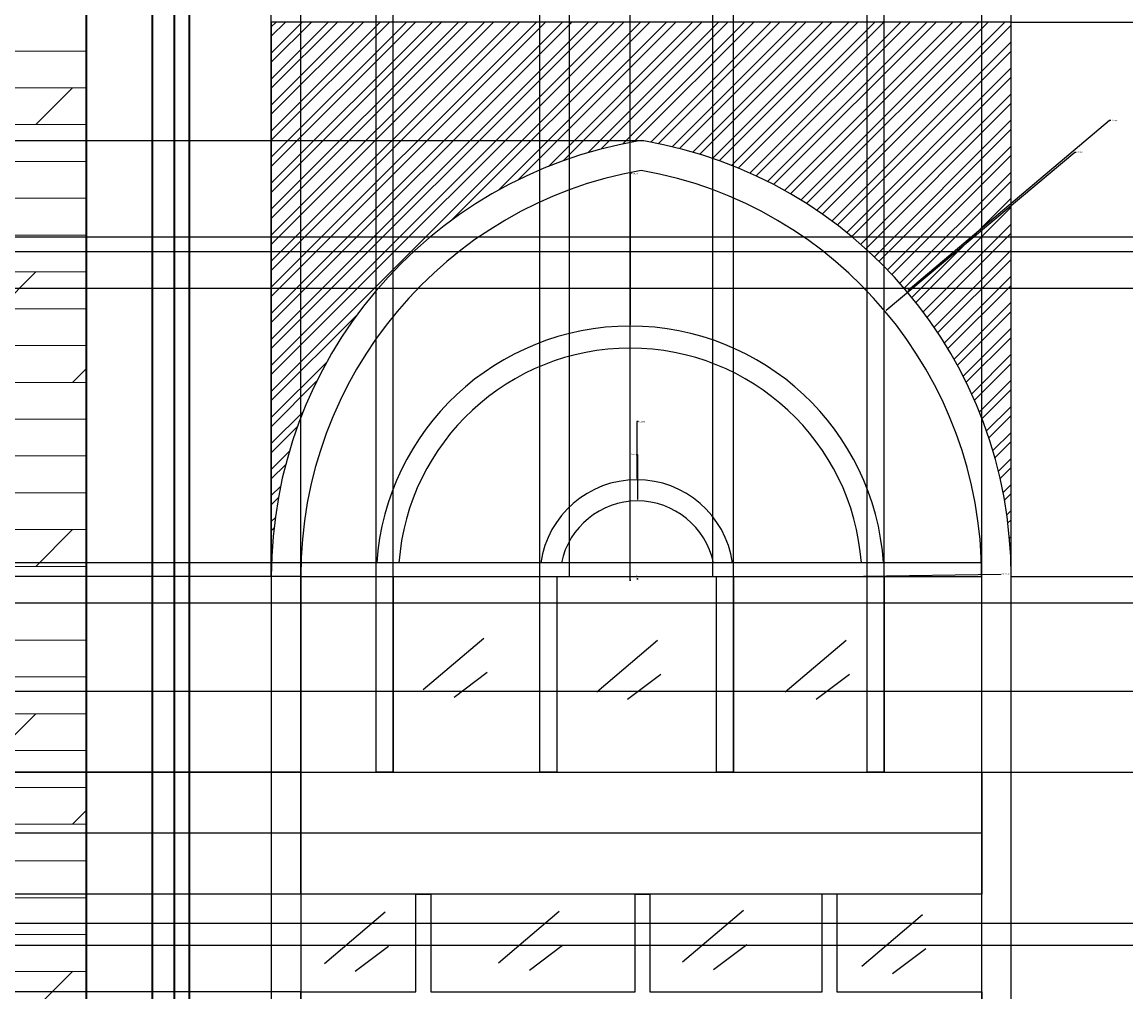
# Model space of a CAD drawing. Units: inches. Extents: x -13 to 630, y -103 to 275.
# Tile 6 of 9: x 168 to 318, y 72 to 204. Entities that reach past the tile are written whole.
import ezdxf

# ---------------------------------------------------------------- set-up
doc = ezdxf.new("R2010")
doc.units = ezdxf.units.IN
doc.header["$MEASUREMENT"] = 0
for name, color, linetype, lineweight in [('A-ANNO-DIMS', 2, 'Continuous', 18), ('A-ELEV', 7, 'Continuous', 35), ('A-ELEV-PATT', 8, 'Continuous', 13), ('A-GLAZ', 4, 'Continuous', 25)]:
    doc.layers.add(name, color=color, linetype=linetype, lineweight=lineweight)
doc.styles.get("Standard").update_dxf_attribs({"font": 'arial.ttf'})
doc.dimstyles.get("Standard").update_dxf_attribs({"dimtxt": 0.18, "dimasz": 0.18, "dimexe": 0.18, "dimexo": 0.0625, "dimgap": 0.09, "dimtad": 0, "dimtih": 1, "dimtoh": 1, "dimdec": 4, "dimzin": 0, "dimdsep": 46, "dimtxsty": 'Standard', "dimcen": 0.09, "dimadec": 0, "dimazin": 0, "dimtfac": 1, "dimtdec": 4, "dimtofl": 0, "dimtmove": 0, "dimatfit": 3, "dimfxl": 1, "dimtolj": 1, "dimtzin": 0, "dimarcsym": 0})

# ---------------------------------------------------------------- blocks, each defined once
blk = doc.blocks.new('GLAZ-MARK')
for p, q in [((0, 1.02), (8.26, 8.03)), ((4.19, 0), (8.71, 3.39))]:
    blk.add_line(p, q)
blk = doc.blocks.new('*D28')
at = {"layer": 'A-ANNO-DIMS', "color": 0, "lineweight": -2, "transparency": 16777216}
for p, q in [((302.59, 128.66), (630.03, 128.66)), ((629.85, 128.48), (629.85, 67.05)), ((629.85, 5.26), (629.85, 66.69)), ((302.59, 5.08), (630.03, 5.08))]:
    blk.add_line(p, q, dxfattribs=at)
at = {"layer": 'A-ANNO-DIMS', "color": 0, "transparency": 16777216}
for points in [[(629.82, 128.48), (629.88, 128.48), (629.85, 128.66)], [(629.82, 5.26), (629.88, 5.26), (629.85, 5.08)]]:
    blk.add_solid(points, dxfattribs=at)
at = {"layer": 'Defpoints', "color": 0, "transparency": 16777216}
for p in [(302.53, 128.66), (629.85, 128.66), (302.53, 5.08)]:
    blk.add_point(p, dxfattribs=at)
at = {"layer": 'A-ANNO-DIMS', "color": 0, "transparency": 16777216, "insert": (629.85, 66.87), "char_height": 0.18, "attachment_point": 5}
blk.add_mtext('\\A1;123.57', dxfattribs=at)
blk = doc.blocks.new('*D29')
at = {"layer": 'A-ANNO-DIMS', "color": 0, "lineweight": -2, "transparency": 16777216}
for p, q in [((302.59, 203.94), (630.03, 203.94)), ((629.85, 203.76), (629.85, 166.48)), ((629.85, 128.84), (629.85, 166.11)), ((302.59, 128.66), (630.03, 128.66))]:
    blk.add_line(p, q, dxfattribs=at)
at = {"layer": 'A-ANNO-DIMS', "color": 0, "transparency": 16777216}
for points in [[(629.82, 203.76), (629.88, 203.76), (629.85, 203.94)], [(629.82, 128.84), (629.88, 128.84), (629.85, 128.66)]]:
    blk.add_solid(points, dxfattribs=at)
at = {"layer": 'Defpoints', "color": 0, "transparency": 16777216}
for p in [(302.53, 203.94), (629.85, 203.94), (302.53, 128.66)]:
    blk.add_point(p, dxfattribs=at)
at = {"layer": 'A-ANNO-DIMS', "color": 0, "transparency": 16777216, "insert": (629.85, 166.3), "char_height": 0.18, "attachment_point": 5}
blk.add_mtext('\\A1;75.28', dxfattribs=at)
blk = doc.blocks.new('*D41')
at = {"layer": 'A-ANNO-DIMS', "color": 0, "lineweight": -2, "transparency": 16777216}
for p, q in [((205.96, 72.22), (-13.22, 72.22)), ((-13.04, 72.04), (-13.04, 71.07)), ((-13.04, 69.73), (-13.04, 70.7)), ((205.96, 69.55), (-13.22, 69.55))]:
    blk.add_line(p, q, dxfattribs=at)
at = {"layer": 'A-ANNO-DIMS', "color": 0, "transparency": 16777216}
for points in [[(-13.07, 72.04), (-13.01, 72.04), (-13.04, 72.22)], [(-13.07, 69.73), (-13.01, 69.73), (-13.04, 69.55)]]:
    blk.add_solid(points, dxfattribs=at)
at = {"layer": 'Defpoints', "color": 0, "transparency": 16777216}
for p in [(-13.04, 72.22), (206.02, 72.22), (206.02, 69.55)]:
    blk.add_point(p, dxfattribs=at)
at = {"layer": 'A-ANNO-DIMS', "color": 0, "transparency": 16777216, "insert": (-13.04, 70.88), "char_height": 0.18, "attachment_point": 5}
blk.add_mtext('\\A1;2.68', dxfattribs=at)
blk = doc.blocks.new('*D42')
at = {"layer": 'A-ANNO-DIMS', "color": 0, "lineweight": -2, "transparency": 16777216}
for p, q in [((205.96, 85.52), (-13.22, 85.52)), ((-13.04, 85.34), (-13.04, 79.05)), ((-13.04, 72.4), (-13.04, 78.69)), ((205.96, 72.22), (-13.22, 72.22))]:
    blk.add_line(p, q, dxfattribs=at)
at = {"layer": 'A-ANNO-DIMS', "color": 0, "transparency": 16777216}
for points in [[(-13.07, 85.34), (-13.01, 85.34), (-13.04, 85.52)], [(-13.07, 72.4), (-13.01, 72.4), (-13.04, 72.22)]]:
    blk.add_solid(points, dxfattribs=at)
at = {"layer": 'Defpoints', "color": 0, "transparency": 16777216}
for p in [(-13.04, 85.52), (206.02, 85.52), (206.02, 72.22)]:
    blk.add_point(p, dxfattribs=at)
at = {"layer": 'A-ANNO-DIMS', "color": 0, "transparency": 16777216, "insert": (-13.04, 78.87), "char_height": 0.18, "attachment_point": 5}
blk.add_mtext('\\A1;13.297', dxfattribs=at)
blk = doc.blocks.new('*D43')
at = {"layer": 'A-ANNO-DIMS', "color": 0, "lineweight": -2, "transparency": 16777216}
for p, q in [((205.96, 93.8), (-13.22, 93.8)), ((-13.04, 93.62), (-13.04, 89.84)), ((-13.04, 85.7), (-13.04, 89.48)), ((205.96, 85.52), (-13.22, 85.52))]:
    blk.add_line(p, q, dxfattribs=at)
at = {"layer": 'A-ANNO-DIMS', "color": 0, "transparency": 16777216}
for points in [[(-13.07, 93.62), (-13.01, 93.62), (-13.04, 93.8)], [(-13.07, 85.7), (-13.01, 85.7), (-13.04, 85.52)]]:
    blk.add_solid(points, dxfattribs=at)
at = {"layer": 'Defpoints', "color": 0, "transparency": 16777216}
for p in [(-13.04, 93.8), (206.02, 93.8), (206.02, 85.52)]:
    blk.add_point(p, dxfattribs=at)
at = {"layer": 'A-ANNO-DIMS', "color": 0, "transparency": 16777216, "insert": (-13.04, 89.66), "char_height": 0.18, "attachment_point": 5}
blk.add_mtext('\\A1;8.28', dxfattribs=at)
blk = doc.blocks.new('*D44')
at = {"layer": 'A-ANNO-DIMS', "color": 0, "lineweight": -2, "transparency": 16777216}
for p, q in [((205.96, 102.08), (-13.22, 102.08)), ((-13.04, 101.9), (-13.04, 98.12)), ((-13.04, 93.98), (-13.04, 97.76)), ((205.96, 93.8), (-13.22, 93.8))]:
    blk.add_line(p, q, dxfattribs=at)
at = {"layer": 'A-ANNO-DIMS', "color": 0, "transparency": 16777216}
for points in [[(-13.07, 101.9), (-13.01, 101.9), (-13.04, 102.08)], [(-13.07, 93.98), (-13.01, 93.98), (-13.04, 93.8)]]:
    blk.add_solid(points, dxfattribs=at)
at = {"layer": 'Defpoints', "color": 0, "transparency": 16777216}
for p in [(-13.04, 102.08), (206.02, 102.08), (206.02, 93.8)]:
    blk.add_point(p, dxfattribs=at)
at = {"layer": 'A-ANNO-DIMS', "color": 0, "transparency": 16777216, "insert": (-13.04, 97.94), "char_height": 0.18, "attachment_point": 5}
blk.add_mtext('\\A1;8.28', dxfattribs=at)
blk = doc.blocks.new('*D45')
at = {"layer": 'A-ANNO-DIMS', "color": 0, "lineweight": -2, "transparency": 16777216}
for p, q in [((205.96, 128.66), (-13.22, 128.66)), ((-13.04, 128.48), (-13.04, 115.55)), ((-13.04, 102.26), (-13.04, 115.19)), ((205.96, 102.08), (-13.22, 102.08))]:
    blk.add_line(p, q, dxfattribs=at)
at = {"layer": 'A-ANNO-DIMS', "color": 0, "transparency": 16777216}
for points in [[(-13.07, 128.48), (-13.01, 128.48), (-13.04, 128.66)], [(-13.07, 102.26), (-13.01, 102.26), (-13.04, 102.08)]]:
    blk.add_solid(points, dxfattribs=at)
at = {"layer": 'Defpoints', "color": 0, "transparency": 16777216}
for p in [(-13.04, 128.66), (206.02, 128.66), (206.02, 102.08)]:
    blk.add_point(p, dxfattribs=at)
at = {"layer": 'A-ANNO-DIMS', "color": 0, "transparency": 16777216, "insert": (-13.04, 115.37), "char_height": 0.18, "attachment_point": 5}
blk.add_mtext('\\A1;26.574', dxfattribs=at)
blk = doc.blocks.new('*D46')
at = {"layer": 'A-ANNO-DIMS', "color": 0, "lineweight": -2, "transparency": 16777216}
for p, q in [((205.96, 130.51), (-13.22, 130.51)), ((-13.04, 130.33), (-13.04, 129.76)), ((-13.04, 128.84), (-13.04, 129.4)), ((205.96, 128.66), (-13.22, 128.66))]:
    blk.add_line(p, q, dxfattribs=at)
at = {"layer": 'A-ANNO-DIMS', "color": 0, "transparency": 16777216}
for points in [[(-13.07, 130.33), (-13.01, 130.33), (-13.04, 130.51)], [(-13.07, 128.84), (-13.01, 128.84), (-13.04, 128.66)]]:
    blk.add_solid(points, dxfattribs=at)
at = {"layer": 'Defpoints', "color": 0, "transparency": 16777216}
for p in [(-13.04, 130.51), (206.02, 130.51), (206.02, 128.66)]:
    blk.add_point(p, dxfattribs=at)
at = {"layer": 'A-ANNO-DIMS', "color": 0, "transparency": 16777216, "insert": (-13.04, 129.58), "char_height": 0.18, "attachment_point": 5}
blk.add_mtext('\\A1;1.854', dxfattribs=at)
blk = doc.blocks.new('*D47')
at = {"layer": 'A-ANNO-DIMS', "color": 0, "lineweight": -2, "transparency": 16777216}
for p, q in [((252.21, 187.83), (-13.22, 187.83)), ((-13.04, 187.65), (-13.04, 159.35)), ((-13.04, 130.69), (-13.04, 158.99)), ((205.96, 130.51), (-13.22, 130.51))]:
    blk.add_line(p, q, dxfattribs=at)
at = {"layer": 'A-ANNO-DIMS', "color": 0, "transparency": 16777216}
for points in [[(-13.07, 187.65), (-13.01, 187.65), (-13.04, 187.83)], [(-13.07, 130.69), (-13.01, 130.69), (-13.04, 130.51)]]:
    blk.add_solid(points, dxfattribs=at)
at = {"layer": 'Defpoints', "color": 0, "transparency": 16777216}
for p in [(-13.04, 187.83), (252.27, 187.83), (206.02, 130.51)]:
    blk.add_point(p, dxfattribs=at)
at = {"layer": 'A-ANNO-DIMS', "color": 0, "transparency": 16777216, "insert": (-13.04, 159.17), "char_height": 0.18, "attachment_point": 5}
blk.add_mtext('\\A1;57.32', dxfattribs=at)
blk = doc.blocks.new('*D56')
at = {"layer": 'A-ANNO-DIMS', "color": 0, "lineweight": -2, "transparency": 16777216}
for p, q in [((206.02, 102.14), (206.02, 275.01)), ((206.2, 274.83), (210.69, 274.83)), ((216.09, 274.83), (211.6, 274.83)), ((216.27, 102.14), (216.27, 275.01))]:
    blk.add_line(p, q, dxfattribs=at)
at = {"layer": 'A-ANNO-DIMS', "color": 0, "transparency": 16777216}
for points in [[(206.2, 274.86), (206.2, 274.8), (206.02, 274.83)], [(216.09, 274.86), (216.09, 274.8), (216.27, 274.83)]]:
    blk.add_solid(points, dxfattribs=at)
at = {"layer": 'Defpoints', "color": 0, "transparency": 16777216}
for p in [(216.27, 274.83), (206.02, 102.08), (216.27, 102.08)]:
    blk.add_point(p, dxfattribs=at)
at = {"layer": 'A-ANNO-DIMS', "color": 0, "transparency": 16777216, "insert": (211.14, 274.83), "char_height": 0.18, "attachment_point": 5}
blk.add_mtext('\\A1;10.246', dxfattribs=at)
blk = doc.blocks.new('*D57')
at = {"layer": 'A-ANNO-DIMS', "color": 0, "lineweight": -2, "transparency": 16777216}
for p, q in [((216.27, 102.14), (216.27, 275.01)), ((216.45, 274.83), (217.02, 274.83)), ((218.38, 274.83), (217.81, 274.83)), ((218.56, 102.14), (218.56, 275.01))]:
    blk.add_line(p, q, dxfattribs=at)
at = {"layer": 'A-ANNO-DIMS', "color": 0, "transparency": 16777216}
for points in [[(216.45, 274.86), (216.45, 274.8), (216.27, 274.83)], [(218.38, 274.86), (218.38, 274.8), (218.56, 274.83)]]:
    blk.add_solid(points, dxfattribs=at)
at = {"layer": 'Defpoints', "color": 0, "transparency": 16777216}
for p in [(218.56, 274.83), (216.27, 102.08), (218.56, 102.08)]:
    blk.add_point(p, dxfattribs=at)
at = {"layer": 'A-ANNO-DIMS', "color": 0, "transparency": 16777216, "insert": (217.42, 274.83), "char_height": 0.18, "attachment_point": 5}
blk.add_mtext('\\A1;2.298', dxfattribs=at)
blk = doc.blocks.new('*D58')
at = {"layer": 'A-ANNO-DIMS', "color": 0, "lineweight": -2, "transparency": 16777216}
for p, q in [((218.56, 102.14), (218.56, 275.01)), ((218.74, 274.83), (228.14, 274.83)), ((238.31, 274.83), (228.91, 274.83)), ((238.49, 102.14), (238.49, 275.01))]:
    blk.add_line(p, q, dxfattribs=at)
at = {"layer": 'A-ANNO-DIMS', "color": 0, "transparency": 16777216}
for points in [[(218.74, 274.86), (218.74, 274.8), (218.56, 274.83)], [(238.31, 274.86), (238.31, 274.8), (238.49, 274.83)]]:
    blk.add_solid(points, dxfattribs=at)
at = {"layer": 'Defpoints', "color": 0, "transparency": 16777216}
for p in [(238.49, 274.83), (218.56, 102.08), (238.49, 102.08)]:
    blk.add_point(p, dxfattribs=at)
at = {"layer": 'A-ANNO-DIMS', "color": 0, "transparency": 16777216, "insert": (228.53, 274.83), "char_height": 0.18, "attachment_point": 5}
blk.add_mtext('\\A1;19.93', dxfattribs=at)
blk = doc.blocks.new('*D59')
at = {"layer": 'A-ANNO-DIMS', "color": 0, "lineweight": -2, "transparency": 16777216}
for p, q in [((238.49, 102.14), (238.49, 275.01)), ((238.67, 274.83), (251.26, 274.83)), ((264.64, 274.83), (252.05, 274.83)), ((264.82, 102.14), (264.82, 275.01))]:
    blk.add_line(p, q, dxfattribs=at)
at = {"layer": 'A-ANNO-DIMS', "color": 0, "transparency": 16777216}
for points in [[(238.67, 274.86), (238.67, 274.8), (238.49, 274.83)], [(264.64, 274.86), (264.64, 274.8), (264.82, 274.83)]]:
    blk.add_solid(points, dxfattribs=at)
at = {"layer": 'Defpoints', "color": 0, "transparency": 16777216}
for p in [(264.82, 274.83), (238.49, 102.08), (264.82, 102.08)]:
    blk.add_point(p, dxfattribs=at)
at = {"layer": 'A-ANNO-DIMS', "color": 0, "transparency": 16777216, "insert": (251.66, 274.83), "char_height": 0.18, "attachment_point": 5}
blk.add_mtext('\\A1;26.32', dxfattribs=at)
blk = doc.blocks.new('*D60')
at = {"layer": 'A-ANNO-DIMS', "color": 0, "lineweight": -2, "transparency": 16777216}
for p, q in [((264.82, 102.14), (264.82, 275.01)), ((265, 274.83), (273.44, 274.83)), ((282.8, 274.83), (274.35, 274.83)), ((282.98, 102.14), (282.98, 275.01))]:
    blk.add_line(p, q, dxfattribs=at)
at = {"layer": 'A-ANNO-DIMS', "color": 0, "transparency": 16777216}
for points in [[(265, 274.86), (265, 274.8), (264.82, 274.83)], [(282.8, 274.86), (282.8, 274.8), (282.98, 274.83)]]:
    blk.add_solid(points, dxfattribs=at)
at = {"layer": 'Defpoints', "color": 0, "transparency": 16777216}
for p in [(282.98, 274.83), (264.82, 102.08), (282.98, 102.08)]:
    blk.add_point(p, dxfattribs=at)
at = {"layer": 'A-ANNO-DIMS', "color": 0, "transparency": 16777216, "insert": (273.9, 274.83), "char_height": 0.18, "attachment_point": 5}
blk.add_mtext('\\A1;18.158', dxfattribs=at)
blk = doc.blocks.new('*D61')
at = {"layer": 'A-ANNO-DIMS', "color": 0, "lineweight": -2, "transparency": 16777216}
for p, q in [((282.98, 102.14), (282.98, 275.01)), ((283.16, 274.83), (283.73, 274.83)), ((285.09, 274.83), (284.52, 274.83)), ((285.27, 102.14), (285.27, 275.01))]:
    blk.add_line(p, q, dxfattribs=at)
at = {"layer": 'A-ANNO-DIMS', "color": 0, "transparency": 16777216}
for points in [[(283.16, 274.86), (283.16, 274.8), (282.98, 274.83)], [(285.09, 274.86), (285.09, 274.8), (285.27, 274.83)]]:
    blk.add_solid(points, dxfattribs=at)
at = {"layer": 'Defpoints', "color": 0, "transparency": 16777216}
for p in [(285.27, 274.83), (282.98, 102.08), (285.27, 102.08)]:
    blk.add_point(p, dxfattribs=at)
at = {"layer": 'A-ANNO-DIMS', "color": 0, "transparency": 16777216, "insert": (284.12, 274.83), "char_height": 0.18, "attachment_point": 5}
blk.add_mtext('\\A1;2.298', dxfattribs=at)
blk = doc.blocks.new('*D62')
at = {"layer": 'A-ANNO-DIMS', "color": 0, "lineweight": -2, "transparency": 16777216}
for p, q in [((285.27, 102.14), (285.27, 275.01)), ((285.45, 274.83), (291.44, 274.83)), ((298.35, 274.83), (292.35, 274.83)), ((298.53, 102.14), (298.53, 275.01))]:
    blk.add_line(p, q, dxfattribs=at)
at = {"layer": 'A-ANNO-DIMS', "color": 0, "transparency": 16777216}
for points in [[(285.45, 274.86), (285.45, 274.8), (285.27, 274.83)], [(298.35, 274.86), (298.35, 274.8), (298.53, 274.83)]]:
    blk.add_solid(points, dxfattribs=at)
at = {"layer": 'Defpoints', "color": 0, "transparency": 16777216}
for p in [(298.53, 274.83), (285.27, 102.08), (298.53, 102.08)]:
    blk.add_point(p, dxfattribs=at)
at = {"layer": 'A-ANNO-DIMS', "color": 0, "transparency": 16777216, "insert": (291.9, 274.83), "char_height": 0.18, "attachment_point": 5}
blk.add_mtext('\\A1;13.253', dxfattribs=at)
blk = doc.blocks.new('*D63')
at = {"layer": 'A-ANNO-DIMS', "color": 0, "lineweight": -2, "transparency": 16777216}
for p, q in [((202.02, 128.72), (202.02, 275.01)), ((202.2, 274.83), (221.81, 274.83)), ((242.35, 274.83), (222.74, 274.83)), ((242.53, 128.72), (242.53, 275.01))]:
    blk.add_line(p, q, dxfattribs=at)
at = {"layer": 'A-ANNO-DIMS', "color": 0, "transparency": 16777216}
for points in [[(202.2, 274.86), (202.2, 274.8), (202.02, 274.83)], [(242.35, 274.86), (242.35, 274.8), (242.53, 274.83)]]:
    blk.add_solid(points, dxfattribs=at)
at = {"layer": 'Defpoints', "color": 0, "transparency": 16777216}
for p in [(242.53, 274.83), (202.02, 128.66), (242.53, 128.66)]:
    blk.add_point(p, dxfattribs=at)
at = {"layer": 'A-ANNO-DIMS', "color": 0, "transparency": 16777216, "insert": (222.27, 274.83), "char_height": 0.18, "attachment_point": 5}
blk.add_mtext('\\A1;40.505', dxfattribs=at)
blk = doc.blocks.new('*D64')
at = {"layer": 'A-ANNO-DIMS', "color": 0, "lineweight": -2, "transparency": 16777216}
for p, q in [((242.53, 128.72), (242.53, 275.01)), ((242.71, 274.83), (246.25, 274.83)), ((250.59, 274.83), (247.04, 274.83)), ((250.77, 128.2), (250.77, 275.01))]:
    blk.add_line(p, q, dxfattribs=at)
at = {"layer": 'A-ANNO-DIMS', "color": 0, "transparency": 16777216}
for points in [[(242.71, 274.86), (242.71, 274.8), (242.53, 274.83)], [(250.59, 274.86), (250.59, 274.8), (250.77, 274.83)]]:
    blk.add_solid(points, dxfattribs=at)
at = {"layer": 'Defpoints', "color": 0, "transparency": 16777216}
for p in [(250.77, 274.83), (242.53, 128.66), (250.77, 128.14)]:
    blk.add_point(p, dxfattribs=at)
at = {"layer": 'A-ANNO-DIMS', "color": 0, "transparency": 16777216, "insert": (246.65, 274.83), "char_height": 0.18, "attachment_point": 5}
blk.add_mtext('\\A1;8.244', dxfattribs=at)
blk = doc.blocks.new('*D65')
at = {"layer": 'A-ANNO-DIMS', "color": 0, "lineweight": -2, "transparency": 16777216}
for p, q in [((250.77, 128.2), (250.77, 275.01)), ((250.95, 274.83), (256.01, 274.83)), ((261.84, 274.83), (256.78, 274.83)), ((262.02, 128.72), (262.02, 275.01))]:
    blk.add_line(p, q, dxfattribs=at)
at = {"layer": 'A-ANNO-DIMS', "color": 0, "transparency": 16777216}
for points in [[(250.95, 274.86), (250.95, 274.8), (250.77, 274.83)], [(261.84, 274.86), (261.84, 274.8), (262.02, 274.83)]]:
    blk.add_solid(points, dxfattribs=at)
at = {"layer": 'Defpoints', "color": 0, "transparency": 16777216}
for p in [(262.02, 274.83), (250.77, 128.14), (262.02, 128.66)]:
    blk.add_point(p, dxfattribs=at)
at = {"layer": 'A-ANNO-DIMS', "color": 0, "transparency": 16777216, "insert": (256.4, 274.83), "char_height": 0.18, "attachment_point": 5}
blk.add_mtext('\\A1;11.25', dxfattribs=at)
blk = doc.blocks.new('*D66')
at = {"layer": 'A-ANNO-DIMS', "color": 0, "lineweight": -2, "transparency": 16777216}
for p, q in [((262.02, 128.72), (262.02, 275.01)), ((262.2, 274.83), (281.81, 274.83)), ((302.35, 274.83), (282.74, 274.83)), ((302.53, 128.72), (302.53, 275.01))]:
    blk.add_line(p, q, dxfattribs=at)
at = {"layer": 'A-ANNO-DIMS', "color": 0, "transparency": 16777216}
for points in [[(262.2, 274.86), (262.2, 274.8), (262.02, 274.83)], [(302.35, 274.86), (302.35, 274.8), (302.53, 274.83)]]:
    blk.add_solid(points, dxfattribs=at)
at = {"layer": 'Defpoints', "color": 0, "transparency": 16777216}
for p in [(302.53, 274.83), (262.02, 128.66), (302.53, 128.66)]:
    blk.add_point(p, dxfattribs=at)
at = {"layer": 'A-ANNO-DIMS', "color": 0, "transparency": 16777216, "insert": (282.27, 274.83), "char_height": 0.18, "attachment_point": 5}
blk.add_mtext('\\A1;40.505', dxfattribs=at)
blk = doc.blocks.new('*D83')
at = {"layer": 'A-ANNO-DIMS', "color": 0, "lineweight": -2, "transparency": 16777216}
for p, q in [((134.77, 78.57), (630.03, 78.57)), ((629.85, 78.39), (629.85, 70.42)), ((629.85, 62.08), (629.85, 70.05)), ((134.77, 61.9), (630.03, 61.9))]:
    blk.add_line(p, q, dxfattribs=at)
at = {"layer": 'A-ANNO-DIMS', "color": 0, "transparency": 16777216}
for points in [[(629.82, 78.39), (629.88, 78.39), (629.85, 78.57)], [(629.82, 62.08), (629.88, 62.08), (629.85, 61.9)]]:
    blk.add_solid(points, dxfattribs=at)
at = {"layer": 'Defpoints', "color": 0, "transparency": 16777216}
for p in [(134.71, 78.57), (629.85, 78.57), (134.71, 61.9)]:
    blk.add_point(p, dxfattribs=at)
at = {"layer": 'A-ANNO-DIMS', "color": 0, "transparency": 16777216, "insert": (629.85, 70.24), "char_height": 0.18, "attachment_point": 5}
blk.add_mtext('\\A1;16.67', dxfattribs=at)
blk = doc.blocks.new('*D84')
at = {"layer": 'A-ANNO-DIMS', "color": 0, "lineweight": -2, "transparency": 16777216}
for p, q in [((137.77, 81.57), (630.03, 81.57)), ((629.85, 81.39), (629.85, 80.25)), ((629.85, 78.75), (629.85, 79.89)), ((134.77, 78.57), (630.03, 78.57))]:
    blk.add_line(p, q, dxfattribs=at)
at = {"layer": 'A-ANNO-DIMS', "color": 0, "transparency": 16777216}
for points in [[(629.82, 81.39), (629.88, 81.39), (629.85, 81.57)], [(629.82, 78.75), (629.88, 78.75), (629.85, 78.57)]]:
    blk.add_solid(points, dxfattribs=at)
at = {"layer": 'Defpoints', "color": 0, "transparency": 16777216}
for p in [(137.71, 81.57), (629.85, 81.57), (134.71, 78.57)]:
    blk.add_point(p, dxfattribs=at)
at = {"layer": 'A-ANNO-DIMS', "color": 0, "transparency": 16777216, "insert": (629.85, 80.07), "char_height": 0.18, "attachment_point": 5}
blk.add_mtext('\\A1;3', dxfattribs=at)
blk = doc.blocks.new('*D85')
at = {"layer": 'A-ANNO-DIMS', "color": 0, "lineweight": -2, "transparency": 16777216}
for p, q in [((137.77, 102.08), (630.03, 102.08)), ((629.85, 101.9), (629.85, 92.01)), ((629.85, 81.75), (629.85, 91.64)), ((137.77, 81.57), (630.03, 81.57))]:
    blk.add_line(p, q, dxfattribs=at)
at = {"layer": 'A-ANNO-DIMS', "color": 0, "transparency": 16777216}
for points in [[(629.82, 101.9), (629.88, 101.9), (629.85, 102.08)], [(629.82, 81.75), (629.88, 81.75), (629.85, 81.57)]]:
    blk.add_solid(points, dxfattribs=at)
at = {"layer": 'Defpoints', "color": 0, "transparency": 16777216}
for p in [(137.71, 102.08), (629.85, 102.08), (137.71, 81.57)]:
    blk.add_point(p, dxfattribs=at)
at = {"layer": 'A-ANNO-DIMS', "color": 0, "transparency": 16777216, "insert": (629.85, 91.83), "char_height": 0.18, "attachment_point": 5}
blk.add_mtext('\\A1;20.51', dxfattribs=at)
blk = doc.blocks.new('*D86')
at = {"layer": 'A-ANNO-DIMS', "color": 0, "lineweight": -2, "transparency": 16777216}
for p, q in [((148.77, 113.08), (630.03, 113.08)), ((629.85, 112.9), (629.85, 107.76)), ((629.85, 102.26), (629.85, 107.4)), ((137.77, 102.08), (630.03, 102.08))]:
    blk.add_line(p, q, dxfattribs=at)
at = {"layer": 'A-ANNO-DIMS', "color": 0, "transparency": 16777216}
for points in [[(629.82, 112.9), (629.88, 112.9), (629.85, 113.08)], [(629.82, 102.26), (629.88, 102.26), (629.85, 102.08)]]:
    blk.add_solid(points, dxfattribs=at)
at = {"layer": 'Defpoints', "color": 0, "transparency": 16777216}
for p in [(148.71, 113.08), (629.85, 113.08), (137.71, 102.08)]:
    blk.add_point(p, dxfattribs=at)
at = {"layer": 'A-ANNO-DIMS', "color": 0, "transparency": 16777216, "insert": (629.85, 107.58), "char_height": 0.18, "attachment_point": 5}
blk.add_mtext('\\A1;11', dxfattribs=at)
blk = doc.blocks.new('*D113')
at = {"layer": 'A-ANNO-DIMS', "color": 0, "lineweight": -2, "transparency": 16777216}
for p, q in [((120.73, 167.79), (630.03, 167.79)), ((629.85, 167.61), (629.85, 146.61)), ((629.85, 125.26), (629.85, 146.25)), ((132.73, 125.08), (630.03, 125.08))]:
    blk.add_line(p, q, dxfattribs=at)
at = {"layer": 'A-ANNO-DIMS', "color": 0, "transparency": 16777216}
for points in [[(629.82, 167.61), (629.88, 167.61), (629.85, 167.79)], [(629.82, 125.26), (629.88, 125.26), (629.85, 125.08)]]:
    blk.add_solid(points, dxfattribs=at)
at = {"layer": 'Defpoints', "color": 0, "transparency": 16777216}
for p in [(120.66, 167.79), (629.85, 167.79), (132.66, 125.08)]:
    blk.add_point(p, dxfattribs=at)
at = {"layer": 'A-ANNO-DIMS', "color": 0, "transparency": 16777216, "insert": (629.85, 146.43), "char_height": 0.18, "attachment_point": 5}
blk.add_mtext('\\A1;42.705', dxfattribs=at)
blk = doc.blocks.new('*D114')
at = {"layer": 'A-ANNO-DIMS', "color": 0, "lineweight": -2, "transparency": 16777216}
for p, q in [((120.73, 172.79), (630.03, 172.79)), ((629.85, 172.61), (629.85, 170.47)), ((629.85, 167.97), (629.85, 170.1)), ((120.73, 167.79), (630.03, 167.79))]:
    blk.add_line(p, q, dxfattribs=at)
at = {"layer": 'A-ANNO-DIMS', "color": 0, "transparency": 16777216}
for points in [[(629.82, 172.61), (629.88, 172.61), (629.85, 172.79)], [(629.82, 167.97), (629.88, 167.97), (629.85, 167.79)]]:
    blk.add_solid(points, dxfattribs=at)
at = {"layer": 'Defpoints', "color": 0, "transparency": 16777216}
for p in [(120.66, 172.79), (629.85, 172.79), (120.66, 167.79)]:
    blk.add_point(p, dxfattribs=at)
at = {"layer": 'A-ANNO-DIMS', "color": 0, "transparency": 16777216, "insert": (629.85, 170.29), "char_height": 0.18, "attachment_point": 5}
blk.add_mtext('\\A1;5', dxfattribs=at)
blk = doc.blocks.new('*D115')
at = {"layer": 'A-ANNO-DIMS', "color": 0, "lineweight": -2, "transparency": 16777216}
for p, q in [((120.73, 174.79), (630.03, 174.79)), ((629.85, 174.61), (629.85, 173.97)), ((120.73, 172.79), (630.03, 172.79)), ((629.85, 172.97), (629.85, 173.6))]:
    blk.add_line(p, q, dxfattribs=at)
at = {"layer": 'A-ANNO-DIMS', "color": 0, "transparency": 16777216}
for points in [[(629.82, 174.61), (629.88, 174.61), (629.85, 174.79)], [(629.82, 172.97), (629.88, 172.97), (629.85, 172.79)]]:
    blk.add_solid(points, dxfattribs=at)
at = {"layer": 'Defpoints', "color": 0, "transparency": 16777216}
for p in [(120.66, 174.79), (629.85, 174.79), (120.66, 172.79)]:
    blk.add_point(p, dxfattribs=at)
at = {"layer": 'A-ANNO-DIMS', "color": 0, "transparency": 16777216, "insert": (629.85, 173.79), "char_height": 0.18, "attachment_point": 5}
blk.add_mtext('\\A1;2', dxfattribs=at)
blk = doc.blocks.new('*D116')
at = {"layer": 'A-ANNO-DIMS', "color": 0, "lineweight": -2, "transparency": 16777216}
for p, q in [((315.89, 190.57), (288.52, 167.47)), ((316.07, 190.57), (315.89, 190.57)), ((242.44, 128.66), (242.62, 128.66)), ((242.53, 128.57), (242.53, 128.75))]:
    blk.add_line(p, q, dxfattribs=at)
at = {"layer": 'A-ANNO-DIMS', "color": 0, "transparency": 16777216}
blk.add_solid([(288.5, 167.49), (288.54, 167.45), (288.38, 167.35)], dxfattribs=at)
at = {"layer": 'Defpoints', "color": 0, "transparency": 16777216}
for p in [(288.38, 167.35), (242.53, 128.66)]:
    blk.add_point(p, dxfattribs=at)
at = {"layer": 'A-ANNO-DIMS', "color": 0, "transparency": 16777216, "insert": (316.57, 190.57), "char_height": 0.18, "attachment_point": 5}
blk.add_mtext('\\A1;2X R60', dxfattribs=at)
blk = doc.blocks.new('*D117')
at = {"layer": 'A-ANNO-DIMS', "color": 0, "lineweight": -2, "transparency": 16777216}
for p, q in [((311.18, 186.23), (285.57, 164.76)), ((311.36, 186.23), (311.18, 186.23)), ((242.44, 128.66), (242.62, 128.66)), ((242.53, 128.57), (242.53, 128.75))]:
    blk.add_line(p, q, dxfattribs=at)
at = {"layer": 'A-ANNO-DIMS', "color": 0, "transparency": 16777216}
blk.add_solid([(285.55, 164.78), (285.59, 164.73), (285.43, 164.64)], dxfattribs=at)
at = {"layer": 'Defpoints', "color": 0, "transparency": 16777216}
for p in [(285.43, 164.64), (242.53, 128.66)]:
    blk.add_point(p, dxfattribs=at)
at = {"layer": 'A-ANNO-DIMS', "color": 0, "transparency": 16777216, "insert": (311.86, 186.23), "char_height": 0.18, "attachment_point": 5}
blk.add_mtext('\\A1;2X R56', dxfattribs=at)
blk = doc.blocks.new('*D118')
at = {"layer": 'A-ANNO-DIMS', "color": 0, "lineweight": -2, "transparency": 16777216}
for p, q in [((250.95, 183.35), (250.77, 183.35)), ((250.77, 183.35), (250.77, 162.82)), ((250.68, 128.14), (250.86, 128.14)), ((250.77, 128.05), (250.77, 128.23))]:
    blk.add_line(p, q, dxfattribs=at)
at = {"layer": 'A-ANNO-DIMS', "color": 0, "transparency": 16777216}
blk.add_solid([(250.74, 162.82), (250.8, 162.82), (250.77, 162.64)], dxfattribs=at)
at = {"layer": 'Defpoints', "color": 0, "transparency": 16777216}
for p in [(250.77, 162.64), (250.77, 128.14)]:
    blk.add_point(p, dxfattribs=at)
at = {"layer": 'A-ANNO-DIMS', "color": 0, "transparency": 16777216, "insert": (251.41, 183.35), "char_height": 0.18, "attachment_point": 5}
blk.add_mtext('\\A1;R34.51', dxfattribs=at)
blk = doc.blocks.new('*D119')
at = {"layer": 'A-ANNO-DIMS', "color": 0, "lineweight": -2, "transparency": 16777216}
for p, q in [((250.68, 128.14), (250.86, 128.14)), ((250.77, 128.05), (250.77, 128.23)), ((301.17, 128.93), (282.45, 128.64))]:
    blk.add_line(p, q, dxfattribs=at)
at = {"layer": 'A-ANNO-DIMS', "color": 0, "transparency": 16777216}
blk.add_solid([(282.45, 128.67), (282.45, 128.61), (282.27, 128.63)], dxfattribs=at)
at = {"layer": 'Defpoints', "color": 0, "transparency": 16777216}
for p in [(250.77, 128.14), (282.27, 128.63)]:
    blk.add_point(p, dxfattribs=at)
at = {"layer": 'A-ANNO-DIMS', "color": 0, "transparency": 16777216, "insert": (301.83, 128.93), "char_height": 0.18, "attachment_point": 5}
blk.add_mtext('\\A1;3X R31.51', dxfattribs=at)
blk = doc.blocks.new('*D120')
at = {"layer": 'A-ANNO-DIMS', "color": 0, "lineweight": -2, "transparency": 16777216}
for p, q in [((251.84, 149.68), (251.66, 149.68)), ((251.66, 149.68), (251.66, 141.96)), ((251.57, 128.62), (251.75, 128.62)), ((251.66, 128.53), (251.66, 128.71))]:
    blk.add_line(p, q, dxfattribs=at)
at = {"layer": 'A-ANNO-DIMS', "color": 0, "transparency": 16777216}
blk.add_solid([(251.63, 141.96), (251.69, 141.96), (251.66, 141.78)], dxfattribs=at)
at = {"layer": 'Defpoints', "color": 0, "transparency": 16777216}
for p in [(251.66, 141.78), (251.66, 128.62)]:
    blk.add_point(p, dxfattribs=at)
at = {"layer": 'A-ANNO-DIMS', "color": 0, "transparency": 16777216, "insert": (252.37, 149.68), "char_height": 0.18, "attachment_point": 5}
blk.add_mtext('\\A1;R13.161', dxfattribs=at)
blk = doc.blocks.new('*D121')
at = {"layer": 'A-ANNO-DIMS', "color": 0, "lineweight": -2, "transparency": 16777216}
for p, q in [((251.57, 145.23), (251.75, 145.23)), ((251.75, 145.23), (251.75, 139.08)), ((251.66, 128.34), (251.84, 128.34)), ((251.75, 128.25), (251.75, 128.43))]:
    blk.add_line(p, q, dxfattribs=at)
at = {"layer": 'A-ANNO-DIMS', "color": 0, "transparency": 16777216}
blk.add_solid([(251.78, 139.08), (251.72, 139.08), (251.75, 138.9)], dxfattribs=at)
at = {"layer": 'Defpoints', "color": 0, "transparency": 16777216}
for p in [(251.75, 138.9), (251.75, 128.34)]:
    blk.add_point(p, dxfattribs=at)
at = {"layer": 'A-ANNO-DIMS', "color": 0, "transparency": 16777216, "insert": (251.02, 145.23), "char_height": 0.18, "attachment_point": 5}
blk.add_mtext('\\A1;R10.553', dxfattribs=at)

msp = doc.modelspace()

# ---------------------------------------------------------------- hatches: boundary and pattern name
at = {"layer": 'A-ELEV-PATT', "transparency": 33554541}
h = msp.add_hatch(dxfattribs=at)
h.set_pattern_fill('DOLMIT', color=256, scale=20)
h.paths.add_polyline_path([(345.3061, 245.0808), (164.8443, 245.0808), (164.8443, 5.0808), (176.8443, 5.0808), (176.8443, 233.0808), (333.3061, 233.0808), (333.3061, 5.0808), (345.3061, 5.0808)])
at = {"layer": 'A-ELEV-PATT'}
h = msp.add_hatch(dxfattribs=at)
h.set_pattern_fill('BRSTONE', color=256, scale=20)
h.paths.add_polyline_path([(120.6641, 172.7854), (64.9953, 172.7854, 0.41421356), (54.9953, 162.7854), (54.9953, 125.0808), (59.9953, 125.0808), (59.9953, 162.7854, -0.41421356), (64.9953, 167.7854), (120.6641, 167.7854, -0.41421356), (125.6641, 162.7854), (125.6641, 125.0808), (130.6641, 125.0808), (130.6641, 162.7854, 0.41421356)])
h.paths.add_polyline_path([(439.5513, 172.7854), (383.8825, 172.7854, 0.41421356), (373.8825, 162.7854), (373.8825, 125.0808), (378.8825, 125.0808), (378.8825, 162.7854, -0.41421356), (383.8825, 167.7854), (439.5513, 167.7854, -0.41421356), (444.5513, 162.7854), (444.5513, 125.0808), (449.5513, 125.0808), (449.5513, 162.7854, 0.41421356)])
h.paths.add_polyline_path([(364.7117, 113.0808), (484.7117, 113.0808), (484.7117, 5.0808), (496.7117, 5.0808), (496.7117, 125.0808), (345.3061, 125.0808), (345.3061, 5.0808), (364.7117, 5.0808)])
h.paths.add_polyline_path([(164.8443, 125.0808), (28.7117, 125.0808), (16.7117, 125.0808), (16.7117, 5.0808), (28.7117, 5.0808), (28.7117, 113.0808), (148.7117, 113.0808), (148.7117, 5.0808), (164.8443, 5.0808)])
h.paths.add_polyline_path([(95.1171, 223.9392), (83.8622, 223.9392), (83.8622, 206.5279), (95.1171, 206.5279)])
h.paths.add_polyline_path([(54.9212, 223.9392), (40.7186, 223.9392), (40.7186, 206.5279), (54.9212, 206.5279)])
h.paths.add_polyline_path([(463.828, 223.9392), (449.6254, 223.9392), (449.6254, 206.5279), (463.828, 206.5279)])
h.paths.add_polyline_path([(420.6843, 223.9392), (409.4295, 223.9392), (409.4295, 206.5279), (420.6843, 206.5279)])
h = msp.add_hatch(dxfattribs=at)
h.set_pattern_fill('STEEL', color=256, scale=20)
h.set_pattern_definition([(45, (0, 0), (-1.767767, 1.767767), []), (45, (0, 1.25), (-1.767767, 1.767767), [])])
h.paths.add_polyline_path([(164.8443, 218.2056), (95.1171, 218.2056), (95.1171, 215.2335), (164.8443, 215.2335)])
h.paths.add_polyline_path([(83.8622, 218.2056), (54.9212, 218.2056), (54.9212, 215.2335), (83.8622, 215.2335)])
h.paths.add_polyline_path([(409.4295, 218.2056), (345.3061, 218.2056), (345.3061, 215.2335), (409.4295, 215.2335)])
h.paths.add_polyline_path([(449.6254, 218.2056), (420.6843, 218.2056), (420.6843, 215.2335), (449.6254, 215.2335)])
h.paths.add_polyline_path([(302.5258, 203.9359), (202.0208, 203.9359), (202.0208, 128.6551, -0.36718729), (252.2733, 187.858, -0.36718729), (302.5258, 128.6551)])

# ---------------------------------------------------------------- linework, layer by layer
at = {"layer": 'A-ELEV'}
for points in [[(333.3061, 5.0808), (333.3061, 233.0808), (176.8443, 233.0808), (176.8443, 5.0808)], [(324.3061, 5.0808), (324.3061, 224.0808), (185.8443, 224.0808), (185.8443, 5.0808)], [(321.3061, 5.0808), (321.3061, 221.0808), (188.8443, 221.0808), (188.8443, 5.0808)], [(319.3061, 5.0808), (319.3061, 219.0808), (190.8443, 219.0808), (190.8443, 5.0808)]]:
    msp.add_lwpolyline(points, dxfattribs=at)
at = {"layer": 'A-GLAZ'}
for p, q in [((302.5258, 203.9359), (202.0208, 203.9359)), ((202.0208, 203.9359), (202.0208, 5.0808)), ((302.5258, 5.0808), (302.5258, 203.9359)), ((206.0208, 128.6551), (206.0208, 5.0808)), ((298.5258, 5.0808), (298.5258, 128.6551))]:
    msp.add_line(p, q, dxfattribs=at)
for points in [[(251.9372, 187.8017, 0.36557664), (202.0208, 128.6551)], [(302.5258, 128.6551, 0.36557664), (252.6094, 187.8017, 0.36557664)], [(298.5258, 128.6551, 0.36385106), (252.2733, 183.8003, 0.36385106), (206.0208, 128.6551, 0.36385106)]]:
    msp.add_lwpolyline(points, format="xyb", dxfattribs=at)
for points in [[(206.0208, 128.6551), (298.4951, 128.6551), (298.4951, 130.5093), (206.0208, 130.5093)], [(216.2667, 128.6551), (218.5646, 128.6551), (218.5646, 102.0808), (216.2667, 102.0808)], [(238.4945, 128.6551), (240.7924, 128.6551), (240.7924, 102.0808), (238.4945, 102.0808)], [(262.5192, 128.6551), (264.8171, 128.6551), (264.8171, 102.0808), (262.5192, 102.0808)], [(282.9751, 128.6551), (285.273, 128.6551), (285.273, 102.0808), (282.9751, 102.0808)], [(206.0208, 102.0808), (298.5258, 102.0808), (298.5258, 85.5202), (206.0208, 85.5202)], [(206.0208, 102.0808), (298.5258, 102.0808), (298.5258, 93.8005), (206.0208, 93.8005)]]:
    msp.add_lwpolyline(points, close=True, dxfattribs=at)
for points in [[(221.6752, 72.223), (221.6752, 85.5202), (223.6752, 85.5202), (223.6752, 72.223)], [(251.4352, 72.223), (251.4352, 85.5202), (253.4352, 85.5202), (253.4352, 72.223)], [(276.858, 72.223), (276.858, 85.5202)], [(278.858, 85.5202), (278.858, 72.223)], [(221.6752, 69.5455), (206.0208, 69.5455), (206.0208, 72.223), (221.6752, 72.223)], [(223.6752, 72.223), (251.4352, 72.223)], [(253.4352, 72.223), (276.858, 72.223)], [(278.858, 72.223), (298.5258, 72.223), (298.5258, 69.5455), (278.858, 69.5455)]]:
    msp.add_lwpolyline(points, dxfattribs=at)
for centre, radius, start, end in [((252.2733, 185.8302), 2, 80.324926, 99.675074), ((250.7699, 128.137), 34.507, 3.942043, 176.057957), ((250.7699, 128.137), 31.507, 4.318073, 175.681927), ((251.6558, 128.6225), 13.1613, 8.241928, 171.758072), ((251.7512, 128.3436), 10.5526, 11.842792, 168.157208), ((250.7699, 128.137), 31.507, 179.057758, 179.139682), ((250.7699, 128.137), 31.507, 0.860318, 0.942242)]:
    msp.add_arc(centre, radius, start, end, dxfattribs=at)

# ---------------------------------------------------------------- block references
for p in [(222.6491, 112.2573), (246.2269, 111.9665), (271.8424, 111.9665), (209.2397, 75.0547), (232.8841, 75.1688), (257.8992, 75.2829), (282.229, 74.7123)]:
    msp.add_blockref('GLAZ-MARK', p, dxfattribs=at)

# ---------------------------------------------------------------- dimensions: what is measured, and where the dimension line sits
at = {"layer": 'A-ANNO-DIMS'}
for base, p1, p2, override, picture, middle in [((242.5258, 274.8308), (202.0208, 128.6551), (242.5258, 128.6551), {"dimdec": 3, "dimlfac": 1, "dimrnd": 0, "dimzin": 0, "dimdsep": 46, "dimlunit": 2}, '*D63', (222.2733, 274.8308)), ((216.2667, 274.8308), (206.0208, 102.0808), (216.2667, 102.0808), {"dimdec": 3, "dimlfac": 1, "dimrnd": 0, "dimzin": 0, "dimdsep": 46, "dimlunit": 2}, '*D56', (211.1438, 274.8308)), ((218.5646, 274.8308), (216.2667, 102.0808), (218.5646, 102.0808), {"dimdec": 3, "dimlfac": 1, "dimrnd": 0, "dimzin": 0, "dimdsep": 46, "dimlunit": 2}, '*D57', (217.4157, 274.8308)), ((238.4945, 274.8308), (218.5646, 102.0808), (238.4945, 102.0808), {"dimdec": 2, "dimlfac": 1, "dimrnd": 0, "dimzin": 0, "dimdsep": 46, "dimlunit": 2}, '*D58', (228.5295, 274.8308)), ((264.8171, 274.8308), (238.4945, 102.0808), (264.8171, 102.0808), {"dimdec": 2, "dimlfac": 1, "dimrnd": 0, "dimzin": 0, "dimdsep": 46, "dimlunit": 2}, '*D59', (251.6558, 274.8308)), ((250.7699, 274.8308), (242.5258, 128.6551), (250.7699, 128.137), {"dimdec": 3, "dimlfac": 1, "dimrnd": 0, "dimzin": 0, "dimdsep": 46, "dimlunit": 2}, '*D64', (246.6478, 274.8308)), ((262.0208, 274.8308), (250.7699, 128.137), (262.0208, 128.6551), {"dimdec": 2, "dimlfac": 1, "dimrnd": 0, "dimzin": 0, "dimdsep": 46, "dimlunit": 2}, '*D65', (256.3953, 274.8308)), ((302.5258, 274.8308), (262.0208, 128.6551), (302.5258, 128.6551), {"dimdec": 3, "dimlfac": 1, "dimrnd": 0, "dimzin": 0, "dimdsep": 46, "dimlunit": 2}, '*D66', (282.2733, 274.8308)), ((282.9751, 274.8308), (264.8171, 102.0808), (282.9751, 102.0808), {"dimdec": 3, "dimlfac": 1, "dimrnd": 0, "dimzin": 0, "dimdsep": 46, "dimlunit": 2}, '*D60', (273.8961, 274.8308)), ((285.273, 274.8308), (282.9751, 102.0808), (285.273, 102.0808), {"dimdec": 3, "dimlfac": 1, "dimrnd": 0, "dimzin": 0, "dimdsep": 46, "dimlunit": 2}, '*D61', (284.1241, 274.8308)), ((298.5258, 274.8308), (285.273, 102.0808), (298.5258, 102.0808), {"dimdec": 3, "dimlfac": 1, "dimrnd": 0, "dimzin": 0, "dimdsep": 46, "dimlunit": 2}, '*D62', (291.8994, 274.8308))]:
    dim = msp.add_linear_dim(base=base, p1=p1, p2=p2, dimstyle='Standard', override=override, dxfattribs=at)
    dim.commit()
    dim.dimension.update_dxf_attribs({"geometry": picture, "text_midpoint": middle})
for base, p1, p2, override, picture, middle in [((629.8508, 203.9359), (302.5258, 128.6551), (302.5258, 203.9359), {"dimdec": 2, "dimlfac": 1, "dimrnd": 0, "dimzin": 0, "dimdsep": 46, "dimlunit": 2}, '*D29', (629.8508, 166.2955)), ((-13.0383, 187.8302), (206.0208, 130.5093), (252.2733, 187.8302), {"dimdec": 2, "dimlfac": 1, "dimrnd": 0, "dimzin": 0, "dimdsep": 46, "dimlunit": 2}, '*D47', (-13.0383, 159.1697)), ((629.8508, 174.7854), (120.6641, 172.7854), (120.6641, 174.7854), {"dimdec": 0, "dimlfac": 1, "dimrnd": 0, "dimzin": 0, "dimdsep": 46, "dimlunit": 2}, '*D115', (629.8508, 173.7854)), ((629.8508, 172.7854), (120.6641, 167.7854), (120.6641, 172.7854), {"dimdec": 0, "dimlfac": 1, "dimrnd": 0, "dimzin": 0, "dimdsep": 46, "dimlunit": 2}, '*D114', (629.8508, 170.2854)), ((629.8508, 167.7854), (132.6641, 125.0808), (120.6641, 167.7854), {"dimdec": 3, "dimlfac": 1, "dimrnd": 0, "dimzin": 0, "dimdsep": 46, "dimlunit": 2}, '*D113', (629.8508, 146.4331)), ((-13.0383, 130.5093), (206.0208, 128.6551), (206.0208, 130.5093), {"dimdec": 3, "dimlfac": 1, "dimrnd": 0, "dimzin": 0, "dimdsep": 46, "dimlunit": 2}, '*D46', (-13.0383, 129.5822)), ((-13.0383, 128.6551), (206.0208, 102.0808), (206.0208, 128.6551), {"dimdec": 3, "dimlfac": 1, "dimrnd": 0, "dimzin": 0, "dimdsep": 46, "dimlunit": 2}, '*D45', (-13.0383, 115.368)), ((629.8508, 128.6551), (302.5258, 5.0808), (302.5258, 128.6551), {"dimdec": 2, "dimlfac": 1, "dimrnd": 0, "dimzin": 0, "dimdsep": 46, "dimlunit": 2}, '*D28', (629.8508, 66.868)), ((629.8508, 113.0808), (137.7117, 102.0808), (148.7117, 113.0808), {"dimdec": 0, "dimlfac": 1, "dimrnd": 0, "dimzin": 0, "dimdsep": 46, "dimlunit": 2}, '*D86', (629.8508, 107.5808)), ((-13.0383, 102.0808), (206.0208, 93.8005), (206.0208, 102.0808), {"dimdec": 2, "dimlfac": 1, "dimrnd": 0, "dimzin": 0, "dimdsep": 46, "dimlunit": 2}, '*D44', (-13.0383, 97.9406)), ((629.8508, 102.0808), (137.7117, 81.5713), (137.7117, 102.0808), {"dimdec": 2, "dimlfac": 1, "dimrnd": 0, "dimzin": 0, "dimdsep": 46, "dimlunit": 2}, '*D85', (629.8508, 91.826)), ((-13.0383, 93.8005), (206.0208, 85.5202), (206.0208, 93.8005), {"dimdec": 2, "dimlfac": 1, "dimrnd": 0, "dimzin": 0, "dimdsep": 46, "dimlunit": 2}, '*D43', (-13.0383, 89.6603)), ((-13.0383, 85.5202), (206.0208, 72.223), (206.0208, 85.5202), {"dimdec": 3, "dimlfac": 1, "dimrnd": 0, "dimzin": 0, "dimdsep": 46, "dimlunit": 2}, '*D42', (-13.0383, 78.8716)), ((629.8508, 81.5713), (134.7117, 78.5713), (137.7117, 81.5713), {"dimdec": 0, "dimlfac": 1, "dimrnd": 0, "dimzin": 0, "dimdsep": 46, "dimlunit": 2}, '*D84', (629.8508, 80.0713)), ((629.8508, 78.5713), (134.7117, 61.902), (134.7117, 78.5713), {"dimdec": 2, "dimlfac": 1, "dimrnd": 0, "dimzin": 0, "dimdsep": 46, "dimlunit": 2}, '*D83', (629.8508, 70.2366)), ((-13.0383, 72.223), (206.0208, 69.5455), (206.0208, 72.223), {"dimdec": 2, "dimlfac": 1, "dimrnd": 0, "dimzin": 0, "dimdsep": 46, "dimlunit": 2}, '*D41', (-13.0383, 70.8842))]:
    dim = msp.add_linear_dim(base=base, p1=p1, p2=p2, angle=90, dimstyle='Standard', override=override, dxfattribs=at)
    dim.commit()
    dim.dimension.update_dxf_attribs({"geometry": picture, "text_midpoint": middle})
for center, mpoint, text, override, picture, middle in [((242.5258, 128.6551), (288.3787, 167.3528), '2X <>', {"dimdec": 0, "dimlfac": 1, "dimrnd": 0, "dimzin": 0, "dimdsep": 46, "dimlunit": 2}, '*D116', (316.5701, 190.5713)), ((242.5258, 128.6551), (285.432, 164.642), '2X <>', {"dimdec": 0, "dimlfac": 1, "dimrnd": 0, "dimzin": 0, "dimdsep": 46, "dimlunit": 2}, '*D117', (311.8556, 186.2341)), ((250.7699, 128.137), (282.273, 128.633), '3X <>', {"dimdec": 2, "dimlfac": 1, "dimrnd": 0, "dimzin": 0, "dimdsep": 46, "dimlunit": 2}, '*D119', (301.1749, 128.9306))]:
    dim = msp.add_radius_dim(center=center, mpoint=mpoint, text=text, dimstyle='Standard', override=override, dxfattribs=at)
    dim.commit()
    dim.dimension.update_dxf_attribs({"geometry": picture, "text_midpoint": middle, "dimtype": 164})
for center, mpoint, override, picture, middle in [((250.7699, 128.137), (250.77, 162.644), {"dimdec": 2, "dimlfac": 1, "dimrnd": 0, "dimzin": 0, "dimdsep": 46, "dimlunit": 2}, '*D118', (251.4125, 183.3483)), ((251.6558, 128.6225), (251.656, 141.7839), {"dimdec": 3, "dimlfac": 1, "dimrnd": 0, "dimzin": 0, "dimdsep": 46, "dimlunit": 2}, '*D120', (252.3685, 149.6807)), ((251.7512, 128.3436), (251.751, 138.8962), {"dimdec": 3, "dimlfac": 1, "dimrnd": 0, "dimzin": 0, "dimdsep": 46, "dimlunit": 2}, '*D121', (251.0211, 145.2277))]:
    dim = msp.add_radius_dim(center=center, mpoint=mpoint, dimstyle='Standard', override=override, dxfattribs=at)
    dim.commit()
    dim.dimension.update_dxf_attribs({"geometry": picture, "text_midpoint": middle, "dimtype": 164})

doc.saveas('drawing.dxf')
